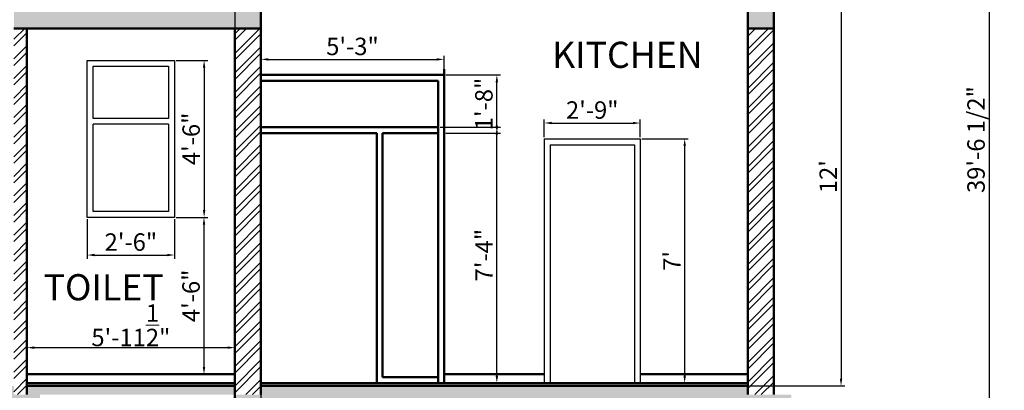
# Model space of a CAD drawing. Units: inches. Extents: x 1615 to 2231, y 1931 to 2519.
# Tile 5 of 6: x 1892 to 2231, y 2153 to 2281. Entities that reach past the tile are written whole.
import ezdxf

# ---------------------------------------------------------------- set-up
doc = ezdxf.new("R2010")
doc.units = ezdxf.units.IN
for name, color, linetype, lineweight in [('A-ANNO-DIMS', 2, 'Continuous', 18), ('A-AREA-IDEN', 7, 'Continuous', 25), ('A-DOOR', 3, 'Continuous', 25), ('A-GLAZ', 4, 'Continuous', 25), ('A-SECT', 7, 'Continuous', 50), ('A-WALL-PATT', 8, 'Continuous', 13)]:
    doc.layers.add(name, color=color, linetype=linetype, lineweight=lineweight)
doc.styles.get("Standard").update_dxf_attribs({"font": 'arial.ttf'})
doc.dimstyles.new('ISO-25', dxfattribs={"dimtxt": 6, "dimasz": 2.5, "dimexe": 1.25, "dimexo": 0.625, "dimtad": 1, "dimdec": 1, "dimlunit": 4, "dimtxsty": 'Standard', "dimcen": 2.5, "dimadec": 0, "dimazin": 0, "dimtfac": 1, "dimtdec": 1, "dimtmove": 0, "dimatfit": 3, "dimfxl": 1, "dimarcsym": 0})

# ---------------------------------------------------------------- blocks, each defined once
blk = doc.blocks.new('*D30')
at = {"layer": 'A-ANNO-DIMS', "color": 0, "lineweight": -2, "transparency": 16777216}
for p, q in [((1915.12, 2211.9), (1915.12, 2198.31)), ((1945.12, 2211.9), (1945.12, 2198.31)), ((1917.62, 2199.56), (1942.62, 2199.56))]:
    blk.add_line(p, q, dxfattribs=at)
at = {"layer": 'A-ANNO-DIMS', "color": 0, "lineweight": 100, "transparency": 16777216}
for points in [[(1917.62, 2199.98), (1917.62, 2199.14), (1915.12, 2199.56)], [(1942.62, 2199.98), (1942.62, 2199.14), (1945.12, 2199.56)]]:
    blk.add_solid(points, dxfattribs=at)
at = {"layer": 'Defpoints', "color": 0, "lineweight": 100, "transparency": 16777216}
for p in [(1915.12, 2212.53), (1945.12, 2212.53), (1945.12, 2199.56)]:
    blk.add_point(p, dxfattribs=at)
at = {"layer": 'A-ANNO-DIMS', "color": 0, "transparency": 16777216, "insert": (1930.12, 2203.25), "char_height": 6, "attachment_point": 5}
blk.add_mtext('2\'-6"', dxfattribs=at)
blk = doc.blocks.new('*D31')
at = {"layer": 'A-ANNO-DIMS', "color": 0, "lineweight": -2, "transparency": 16777216}
for p, q in [((1945.74, 2266.53), (1956.57, 2266.53)), ((1955.32, 2264.03), (1955.32, 2215.03)), ((1945.74, 2212.53), (1956.57, 2212.53))]:
    blk.add_line(p, q, dxfattribs=at)
at = {"layer": 'A-ANNO-DIMS', "color": 0, "lineweight": 100, "transparency": 16777216}
for points in [[(1954.91, 2264.03), (1955.74, 2264.03), (1955.32, 2266.53)], [(1954.91, 2215.03), (1955.74, 2215.03), (1955.32, 2212.53)]]:
    blk.add_solid(points, dxfattribs=at)
at = {"layer": 'Defpoints', "color": 0, "lineweight": 100, "transparency": 16777216}
for p in [(1945.12, 2266.53), (1945.12, 2212.53), (1955.32, 2212.53)]:
    blk.add_point(p, dxfattribs=at)
at = {"layer": 'A-ANNO-DIMS', "color": 0, "transparency": 16777216, "insert": (1951.63, 2239.53), "char_height": 6, "attachment_point": 5, "rotation": 90}
blk.add_mtext('4\'-6"', dxfattribs=at)
blk = doc.blocks.new('*D32')
at = {"layer": 'A-ANNO-DIMS', "color": 0, "lineweight": -2, "transparency": 16777216}
for p, q in [((1945.74, 2212.53), (1956.53, 2212.53)), ((1955.28, 2210.03), (1955.28, 2161.03)), ((1945.74, 2158.53), (1956.53, 2158.53))]:
    blk.add_line(p, q, dxfattribs=at)
at = {"layer": 'A-ANNO-DIMS', "color": 0, "lineweight": 100, "transparency": 16777216}
for points in [[(1954.87, 2210.03), (1955.7, 2210.03), (1955.28, 2212.53)], [(1954.87, 2161.03), (1955.7, 2161.03), (1955.28, 2158.53)]]:
    blk.add_solid(points, dxfattribs=at)
at = {"layer": 'Defpoints', "color": 0, "lineweight": 100, "transparency": 16777216}
for p in [(1945.12, 2212.53), (1945.12, 2158.53), (1955.28, 2158.53)]:
    blk.add_point(p, dxfattribs=at)
at = {"layer": 'A-ANNO-DIMS', "color": 0, "transparency": 16777216, "insert": (1951.6, 2185.53), "char_height": 6, "attachment_point": 5, "rotation": 90}
blk.add_mtext('4\'-6"', dxfattribs=at)
blk = doc.blocks.new('*D44')
at = {"layer": 'A-ANNO-DIMS', "color": 0, "lineweight": -2, "transparency": 16777216}
for p, q in [((2036.49, 2243.53), (2057.3, 2243.53)), ((2056.05, 2158.03), (2056.05, 2241.03)), ((2038.49, 2155.53), (2057.3, 2155.53))]:
    blk.add_line(p, q, dxfattribs=at)
at = {"layer": 'A-ANNO-DIMS', "color": 0, "lineweight": 100, "transparency": 16777216}
for points in [[(2055.63, 2241.03), (2056.47, 2241.03), (2056.05, 2243.53)], [(2055.63, 2158.03), (2056.47, 2158.03), (2056.05, 2155.53)]]:
    blk.add_solid(points, dxfattribs=at)
at = {"layer": 'Defpoints', "color": 0, "lineweight": 100, "transparency": 16777216}
for p in [(2035.87, 2243.53), (2056.05, 2243.53), (2037.87, 2155.53)]:
    blk.add_point(p, dxfattribs=at)
at = {"layer": 'A-ANNO-DIMS', "color": 0, "transparency": 16777216, "insert": (2052.43, 2199.53), "char_height": 6, "attachment_point": 5, "rotation": 90}
blk.add_mtext('7\'-4"', dxfattribs=at)
blk = doc.blocks.new('*D45')
at = {"layer": 'A-ANNO-DIMS', "color": 0, "lineweight": -2, "transparency": 16777216}
for p, q in [((1974.87, 2262.15), (1974.87, 2268.12)), ((1977.37, 2266.87), (2035.37, 2266.87)), ((2037.87, 2262.15), (2037.87, 2268.12))]:
    blk.add_line(p, q, dxfattribs=at)
at = {"layer": 'A-ANNO-DIMS', "color": 0, "lineweight": 100, "transparency": 16777216}
for points in [[(1977.37, 2267.29), (1977.37, 2266.46), (1974.87, 2266.87)], [(2035.37, 2267.29), (2035.37, 2266.46), (2037.87, 2266.87)]]:
    blk.add_solid(points, dxfattribs=at)
at = {"layer": 'Defpoints', "color": 0, "lineweight": 100, "transparency": 16777216}
for p in [(2037.87, 2266.87), (1974.87, 2261.53), (2037.87, 2261.53)]:
    blk.add_point(p, dxfattribs=at)
at = {"layer": 'A-ANNO-DIMS', "color": 0, "transparency": 16777216, "insert": (2006.37, 2270.56), "char_height": 6, "attachment_point": 5}
blk.add_mtext('5\'-3"', dxfattribs=at)
blk = doc.blocks.new('*D49')
at = {"layer": 'A-ANNO-DIMS', "color": 0, "lineweight": -2, "transparency": 16777216}
for p, q in [((2038.49, 2261.53), (2057.3, 2261.53)), ((2056.05, 2244.03), (2056.05, 2259.03)), ((2038.49, 2241.53), (2057.3, 2241.53))]:
    blk.add_line(p, q, dxfattribs=at)
at = {"layer": 'A-ANNO-DIMS', "color": 0, "lineweight": 100, "transparency": 16777216}
for points in [[(2055.63, 2259.03), (2056.47, 2259.03), (2056.05, 2261.53)], [(2055.63, 2244.03), (2056.47, 2244.03), (2056.05, 2241.53)]]:
    blk.add_solid(points, dxfattribs=at)
at = {"layer": 'Defpoints', "color": 0, "lineweight": 100, "transparency": 16777216}
for p in [(2037.87, 2261.53), (2056.05, 2261.53), (2037.87, 2241.53)]:
    blk.add_point(p, dxfattribs=at)
at = {"layer": 'A-ANNO-DIMS', "color": 0, "transparency": 16777216, "insert": (2052.36, 2251.53), "char_height": 6, "attachment_point": 5, "rotation": 90}
blk.add_mtext('1\'-8"', dxfattribs=at)
blk = doc.blocks.new('*D50')
at = {"layer": 'A-ANNO-DIMS', "color": 0, "lineweight": -2, "transparency": 16777216}
for p, q in [((1974.87, 2262.15), (1974.87, 2268.12)), ((1977.37, 2266.87), (2035.37, 2266.87)), ((2037.87, 2262.15), (2037.87, 2268.12))]:
    blk.add_line(p, q, dxfattribs=at)
at = {"layer": 'A-ANNO-DIMS', "color": 0, "lineweight": 100, "transparency": 16777216}
for points in [[(1977.37, 2267.29), (1977.37, 2266.46), (1974.87, 2266.87)], [(2035.37, 2267.29), (2035.37, 2266.46), (2037.87, 2266.87)]]:
    blk.add_solid(points, dxfattribs=at)
at = {"layer": 'Defpoints', "color": 0, "lineweight": 100, "transparency": 16777216}
for p in [(2037.87, 2266.87), (1974.87, 2261.53), (2037.87, 2261.53)]:
    blk.add_point(p, dxfattribs=at)
at = {"layer": 'A-ANNO-DIMS', "color": 0, "transparency": 16777216, "insert": (2006.37, 2270.56), "char_height": 6, "attachment_point": 5}
blk.add_mtext('5\'-3"', dxfattribs=at)
blk = doc.blocks.new('*D51')
at = {"layer": 'A-ANNO-DIMS', "color": 0, "lineweight": -2, "transparency": 16777216}
for p, q in [((2105.99, 2239.53), (2121.93, 2239.53)), ((2120.68, 2158.03), (2120.68, 2237.03)), ((2105.99, 2155.53), (2121.93, 2155.53))]:
    blk.add_line(p, q, dxfattribs=at)
at = {"layer": 'A-ANNO-DIMS', "color": 0, "lineweight": 100, "transparency": 16777216}
for points in [[(2120.27, 2237.03), (2121.1, 2237.03), (2120.68, 2239.53)], [(2120.27, 2158.03), (2121.1, 2158.03), (2120.68, 2155.53)]]:
    blk.add_solid(points, dxfattribs=at)
at = {"layer": 'Defpoints', "color": 0, "lineweight": 100, "transparency": 16777216}
for p in [(2105.37, 2239.53), (2120.68, 2239.53), (2105.37, 2155.53)]:
    blk.add_point(p, dxfattribs=at)
at = {"layer": 'A-ANNO-DIMS', "color": 0, "transparency": 16777216, "insert": (2117.06, 2197.53), "char_height": 6, "attachment_point": 5, "rotation": 90}
blk.add_mtext("7'", dxfattribs=at)
blk = doc.blocks.new('*D52')
at = {"layer": 'A-ANNO-DIMS', "color": 0, "lineweight": -2, "transparency": 16777216}
for p, q in [((2072.37, 2240.15), (2072.37, 2246.23)), ((2105.37, 2240.15), (2105.37, 2246.23)), ((2074.87, 2244.98), (2102.87, 2244.98))]:
    blk.add_line(p, q, dxfattribs=at)
at = {"layer": 'A-ANNO-DIMS', "color": 0, "lineweight": 100, "transparency": 16777216}
for points in [[(2074.87, 2245.4), (2074.87, 2244.57), (2072.37, 2244.98)], [(2102.87, 2245.4), (2102.87, 2244.57), (2105.37, 2244.98)]]:
    blk.add_solid(points, dxfattribs=at)
at = {"layer": 'Defpoints', "color": 0, "lineweight": 100, "transparency": 16777216}
for p in [(2105.37, 2244.98), (2072.37, 2239.53), (2105.37, 2239.53)]:
    blk.add_point(p, dxfattribs=at)
at = {"layer": 'A-ANNO-DIMS', "color": 0, "transparency": 16777216, "insert": (2088.87, 2248.67), "char_height": 6, "attachment_point": 5}
blk.add_mtext('2\'-9"', dxfattribs=at)
blk = doc.blocks.new('*D53')
at = {"layer": 'A-ANNO-DIMS', "color": 0, "lineweight": -2, "transparency": 16777216}
for p, q in [((2036.49, 2243.53), (2057.3, 2243.53)), ((2056.05, 2158.03), (2056.05, 2241.03)), ((2038.49, 2155.53), (2057.3, 2155.53))]:
    blk.add_line(p, q, dxfattribs=at)
at = {"layer": 'A-ANNO-DIMS', "color": 0, "lineweight": 100, "transparency": 16777216}
for points in [[(2055.63, 2241.03), (2056.47, 2241.03), (2056.05, 2243.53)], [(2055.63, 2158.03), (2056.47, 2158.03), (2056.05, 2155.53)]]:
    blk.add_solid(points, dxfattribs=at)
at = {"layer": 'Defpoints', "color": 0, "lineweight": 100, "transparency": 16777216}
for p in [(2035.87, 2243.53), (2056.05, 2243.53), (2037.87, 2155.53)]:
    blk.add_point(p, dxfattribs=at)
at = {"layer": 'A-ANNO-DIMS', "color": 0, "transparency": 16777216, "insert": (2052.43, 2199.53), "char_height": 6, "attachment_point": 5, "rotation": 90}
blk.add_mtext('7\'-4"', dxfattribs=at)
blk = doc.blocks.new('*D60')
at = {"layer": 'A-ANNO-DIMS', "color": 0, "lineweight": -2, "transparency": 16777216}
for p, q in [((1894.37, 2159.15), (1894.37, 2168.95)), ((1965.87, 2159.15), (1965.87, 2168.95)), ((1896.87, 2167.7), (1963.37, 2167.7))]:
    blk.add_line(p, q, dxfattribs=at)
at = {"layer": 'A-ANNO-DIMS', "color": 0, "lineweight": 100, "transparency": 16777216}
for points in [[(1896.87, 2168.12), (1896.87, 2167.28), (1894.37, 2167.7)], [(1963.37, 2168.12), (1963.37, 2167.28), (1965.87, 2167.7)]]:
    blk.add_solid(points, dxfattribs=at)
at = {"layer": 'Defpoints', "color": 0, "lineweight": 100, "transparency": 16777216}
for p in [(1965.87, 2167.7), (1894.37, 2158.53), (1965.87, 2158.53)]:
    blk.add_point(p, dxfattribs=at)
at = {"layer": 'A-ANNO-DIMS', "color": 0, "transparency": 16777216, "insert": (1930.12, 2175.4), "char_height": 6, "attachment_point": 5}
blk.add_mtext('5\'-11{\\H1x;\\S1/2;}"', dxfattribs=at)
blk = doc.blocks.new('*D63')
at = {"layer": 'A-ANNO-DIMS', "color": 0, "lineweight": -2, "transparency": 16777216}
for p, q in [((2142.99, 2298.53), (2175.73, 2298.53)), ((2174.48, 2296.03), (2174.48, 2157.03)), ((2142.99, 2154.53), (2175.73, 2154.53))]:
    blk.add_line(p, q, dxfattribs=at)
at = {"layer": 'A-ANNO-DIMS', "color": 0, "lineweight": 100, "transparency": 16777216}
for points in [[(2174.07, 2296.03), (2174.9, 2296.03), (2174.48, 2298.53)], [(2174.07, 2157.03), (2174.9, 2157.03), (2174.48, 2154.53)]]:
    blk.add_solid(points, dxfattribs=at)
at = {"layer": 'Defpoints', "color": 0, "lineweight": 100, "transparency": 16777216}
for p in [(2142.37, 2298.53), (2142.37, 2154.53), (2174.48, 2154.53)]:
    blk.add_point(p, dxfattribs=at)
at = {"layer": 'A-ANNO-DIMS', "color": 0, "transparency": 16777216, "insert": (2170.85, 2226.53), "char_height": 6, "attachment_point": 5, "rotation": 90}
blk.add_mtext("12'", dxfattribs=at)
blk = doc.blocks.new('WIN-TOILET')
for p, q in [((1915.12, 2410.53), (1945.12, 2410.53)), ((1915.12, 2356.53), (1915.12, 2410.53)), ((1945.12, 2410.53), (1945.12, 2390.53)), ((1917.12, 2408.53), (1943.12, 2408.53)), ((1917.12, 2390.53), (1917.12, 2408.53)), ((1943.12, 2408.53), (1943.12, 2390.53)), ((1943.12, 2390.53), (1917.12, 2390.53)), ((1943.12, 2388.53), (1917.12, 2388.53)), ((1917.12, 2358.53), (1917.12, 2388.53)), ((1943.12, 2388.53), (1943.12, 2358.53)), ((1945.12, 2390.53), (1945.12, 2356.53)), ((1943.12, 2358.53), (1917.12, 2358.53)), ((1945.12, 2356.53), (1915.12, 2356.53))]:
    blk.add_line(p, q)
blk = doc.blocks.new('DOOR-KITCHEN')
for p, q in [((2072.37, 2383.53), (2072.37, 2299.53)), ((2072.37, 2383.53), (2105.37, 2383.53)), ((2105.37, 2383.53), (2105.37, 2299.53)), ((2074.37, 2381.53), (2103.37, 2381.53)), ((2074.37, 2381.53), (2074.37, 2299.53)), ((2103.37, 2381.53), (2103.37, 2299.53))]:
    blk.add_line(p, q)
blk = doc.blocks.new('*D79')
at = {"layer": 'A-ANNO-DIMS', "color": 0, "lineweight": -2, "transparency": 16777216}
for p, q in [((2151.99, 2476.53), (2226.69, 2476.53)), ((2225.44, 2474.03), (2225.44, 2004.53)), ((2175.99, 2002.03), (2226.69, 2002.03))]:
    blk.add_line(p, q, dxfattribs=at)
at = {"layer": 'A-ANNO-DIMS', "color": 0, "lineweight": 100, "transparency": 16777216}
for points in [[(2225.02, 2474.03), (2225.86, 2474.03), (2225.44, 2476.53)], [(2225.02, 2004.53), (2225.86, 2004.53), (2225.44, 2002.03)]]:
    blk.add_solid(points, dxfattribs=at)
at = {"layer": 'Defpoints', "color": 0, "lineweight": 100, "transparency": 16777216}
for p in [(2151.37, 2476.53), (2175.37, 2002.03), (2225.44, 2002.03)]:
    blk.add_point(p, dxfattribs=at)
at = {"layer": 'A-ANNO-DIMS', "color": 0, "transparency": 16777216, "insert": (2221.71, 2239.28), "char_height": 6, "attachment_point": 5, "rotation": 90}
blk.add_mtext('39\'-6 1/2"', dxfattribs=at)
blk = doc.blocks.new('*D83')
at = {"layer": 'A-ANNO-DIMS', "color": 0, "lineweight": -2, "transparency": 16777216}
for p, q in [((1965.87, 2420.67), (1965.87, 1970.95)), ((1974.87, 2420.67), (1974.87, 1970.95)), ((1968.37, 1972.2), (1972.37, 1972.2)), ((1974.87, 1972.2), (1994.57, 1972.2))]:
    blk.add_line(p, q, dxfattribs=at)
at = {"layer": 'A-ANNO-DIMS', "color": 0, "lineweight": 100, "transparency": 16777216}
for points in [[(1968.37, 1972.62), (1968.37, 1971.78), (1965.87, 1972.2)], [(1972.37, 1972.62), (1972.37, 1971.78), (1974.87, 1972.2)]]:
    blk.add_solid(points, dxfattribs=at)
at = {"layer": 'Defpoints', "color": 0, "lineweight": 100, "transparency": 16777216}
for p in [(1965.87, 2421.29), (1974.87, 2421.29), (1974.87, 1972.2)]:
    blk.add_point(p, dxfattribs=at)
at = {"layer": 'A-ANNO-DIMS', "color": 0, "transparency": 16777216, "insert": (1985.97, 1975.89), "char_height": 6, "attachment_point": 5}
blk.add_mtext('0\'-9"', dxfattribs=at)

msp = doc.modelspace()

# ---------------------------------------------------------------- hatches: boundary and pattern name
at = {"layer": 'A-WALL-PATT'}
h = msp.add_hatch(dxfattribs=at)
h.set_pattern_fill('ANSI32', color=256, scale=0.5)
h.paths.add_polyline_path([(1676.87, 2421.53), (1667.87, 2421.53), (1667.87, 2295.53), (1676.87, 2295.53)])
h.paths.add_polyline_path([(1676.87, 2277.53), (1667.87, 2277.53), (1667.87, 2151.53), (1676.87, 2151.53)])
h.paths.add_polyline_path([(1676.87, 2476.53), (1667.87, 2476.53), (1667.87, 2439.53), (1676.87, 2439.53)])
h.paths.add_polyline_path([(1894.37, 2421.29), (1889.87, 2421.29), (1889.87, 2295.53), (1894.37, 2295.53)])
h.paths.add_polyline_path([(1974.87, 2421.29), (1965.87, 2421.29), (1965.87, 2295.53), (1974.87, 2295.53)])
h.paths.add_polyline_path([(2151.37, 2421.29), (2142.37, 2421.29), (2142.37, 2295.53), (2151.37, 2295.53)])
h.paths.add_polyline_path([(2151.37, 2476.53), (2142.37, 2476.53), (2142.37, 2442.53), (2151.37, 2442.53)])
h.paths.add_polyline_path([(1974.87, 2277.53), (1965.87, 2277.53), (1965.87, 2151.53), (1974.87, 2151.53)])
h.paths.add_polyline_path([(1974.87, 2133.53), (1965.87, 2133.53), (1965.87, 2060.03), (1974.87, 2060.03)])
h.paths.add_polyline_path([(2098.87, 2145.53), (2094.37, 2145.53), (2094.37, 2059.03), (2098.87, 2059.03)])
h = msp.add_hatch(dxfattribs=at)
h.set_pattern_fill('AR-CONC', color=256, scale=0.1)
h.paths.add_polyline_path([(1898.87, 2151.53), (1667.87, 2151.53), (1667.87, 2145.53), (1679.87, 2145.53), (1682.87, 2145.53), (1889.87, 2145.53), (1889.87, 2133.53), (1974.87, 2133.53), (1974.87, 2145.53), (2142.37, 2145.53), (2142.37, 2133.53), (2157.37, 2133.53), (2157.37, 2151.53), (2155.87, 2151.53), (2151.37, 2151.53), (1965.87, 2151.53), (1965.87, 2139.53), (1898.87, 2139.53)])
h.paths.add_polyline_path([(1898.87, 2295.53), (1667.87, 2295.53), (1667.87, 2277.53), (1676.87, 2277.53), (1676.87, 2289.53), (1889.87, 2289.53), (1889.87, 2277.53), (1974.87, 2277.53), (1974.87, 2289.53), (2142.37, 2289.53), (2142.37, 2277.53), (2151.37, 2277.53), (2151.37, 2295.53), (1965.87, 2295.53), (1965.87, 2283.53), (1898.87, 2283.53)])
h.paths.add_polyline_path([(2142.37, 2439.53), (1676.87, 2439.53), (1667.87, 2439.53), (1667.87, 2421.53), (1676.87, 2421.53), (1676.87, 2433.53), (1889.87, 2433.53), (1889.87, 2421.29), (1898.87, 2421.29), (1898.87, 2433.53), (1965.87, 2433.53), (1965.87, 2421.29), (1974.87, 2421.29), (1974.87, 2433.53), (2142.37, 2433.53)])
h = msp.add_hatch(dxfattribs=at)
h.set_pattern_fill('DOTS', color=256, scale=0.5)
h.paths.add_polyline_path([(2142.37, 2442.53), (1839.37, 2442.53), (1676.87, 2442.53), (1676.87, 2439.53), (2142.37, 2439.53)])
h.paths.add_polyline_path([(1889.87, 2298.53), (1676.87, 2298.53), (1676.87, 2295.53), (1889.87, 2295.53)])
h.paths.add_polyline_path([(2142.37, 2298.53), (1974.87, 2298.53), (1974.87, 2295.53), (2142.37, 2295.53)])
h.paths.add_polyline_path([(1889.87, 2154.53), (1676.87, 2154.53), (1676.87, 2151.53), (1889.87, 2151.53)])
h.paths.add_polyline_path([(1965.87, 2154.53), (1894.37, 2154.53), (1894.37, 2151.53), (1965.87, 2151.53)])
h.paths.add_polyline_path([(2142.37, 2154.53), (1974.87, 2154.53), (1974.87, 2151.53), (2142.37, 2151.53)])
h.paths.add_polyline_path([(2094.37, 2062.03), (1974.87, 2062.03), (1974.87, 2059.03), (2094.37, 2059.03)])
h.paths.add_polyline_path([(2142.37, 2062.03), (2098.87, 2062.03), (2098.87, 2059.03), (2142.37, 2059.03)])
h.paths.add_polyline_path([(1956.87, 2049.53), (1693.37, 2049.53), (1693.37, 2046.53), (1956.87, 2046.53)])
h = msp.add_hatch(dxfattribs=at)
h.set_pattern_fill('ANSI32', color=256, scale=0.5)
h.paths.add_polyline_path([(2151.37, 2277.53), (2142.37, 2277.53), (2142.37, 2151.53), (2151.37, 2151.53)])
h.paths.add_polyline_path([(1894.37, 2277.53), (1889.87, 2277.53), (1889.87, 2151.53), (1894.37, 2151.53)])

# ---------------------------------------------------------------- linework, layer by layer
at = {"layer": 'A-SECT'}
for p, q in [((2151.37, 2476.53), (2151.37, 2151.53)), ((1974.87, 2289.53), (1974.87, 2151.53)), ((2142.37, 2289.53), (2142.37, 2151.53)), ((1889.87, 2277.53), (1974.87, 2277.53)), ((1894.37, 2277.53), (1894.37, 2151.53)), ((1965.87, 2277.53), (1965.87, 2139.53)), ((2142.37, 2277.53), (2151.37, 2277.53)), ((2037.87, 2263.53), (2037.87, 2155.53)), ((1974.87, 2261.53), (2037.87, 2261.53)), ((1974.87, 2259.53), (2035.87, 2259.53)), ((2035.87, 2259.53), (2035.87, 2241.53)), ((1974.87, 2243.53), (2035.87, 2243.53)), ((1974.87, 2241.53), (2014.71, 2241.53)), ((2014.71, 2241.53), (2014.71, 2155.53)), ((2016.71, 2241.53), (2016.71, 2157.53)), ((2016.71, 2241.53), (2035.87, 2241.53)), ((2035.87, 2241.53), (2035.87, 2155.53)), ((1894.37, 2158.53), (1965.87, 2158.53)), ((2037.87, 2158.53), (2072.37, 2158.53)), ((2105.37, 2158.53), (2142.37, 2158.53)), ((1894.37, 2155.53), (1965.87, 2155.53)), ((1974.87, 2155.53), (2142.37, 2155.53)), ((2016.71, 2157.53), (2035.87, 2157.53)), ((1894.37, 2154.53), (1965.87, 2154.53)), ((1974.87, 2154.53), (2142.37, 2154.53))]:
    msp.add_line(p, q, dxfattribs=at)

# ---------------------------------------------------------------- block references
at = {"layer": 'A-DOOR'}
msp.add_blockref('DOOR-KITCHEN', (0, -144), dxfattribs=at)
at = {"layer": 'A-GLAZ'}
msp.add_blockref('WIN-TOILET', (0, -144), dxfattribs=at)

# ---------------------------------------------------------------- texts
at = {"layer": 'A-AREA-IDEN', "char_height": 9, "attachment_point": 1}
for s, width, insert in [('KITCHEN', 1.5481, (2075.08, 2272.94)), ('TOILET', 1.0394, (1900.1, 2192.98))]:
    msp.add_mtext_dynamic_manual_height_columns(s, width=width, gutter_width=12.5, heights=[0], dxfattribs=dict(at, insert=insert))

# ---------------------------------------------------------------- dimensions: what is measured, and where the dimension line sits
at = {"layer": 'A-ANNO-DIMS'}
for base, p1, p2, override, picture, middle in [((2225.44, 2002.03), (2151.37, 2476.53), (2175.37, 2002.03), {"dimdec": 1, "dimlfac": 1, "dimrnd": 0, "dimzin": 1, "dimdsep": 46, "dimlunit": 4, "dimfrac": 2}, '*D79', (2221.71, 2239.28)), ((2174.48, 2154.53), (2142.37, 2298.53), (2142.37, 2154.53), {"dimclrd": 0, "dimclre": 0, "dimclrt": 0}, '*D63', (2170.85, 2226.53)), ((1955.32, 2212.53), (1945.12, 2266.53), (1945.12, 2212.53), {"dimclrd": 0, "dimclre": 0, "dimclrt": 0}, '*D31', (1951.63, 2239.53)), ((2056.05, 2261.53), (2037.87, 2241.53), (2037.87, 2261.53), {"dimclrd": 0, "dimclre": 0, "dimclrt": 0}, '*D49', (2052.36, 2251.53)), ((2056.05, 2243.53), (2037.87, 2155.53), (2035.87, 2243.53), {"dimclrd": 0, "dimclre": 0, "dimclrt": 0}, '*D44', (2052.43, 2199.53)), ((2056.05, 2243.53), (2037.87, 2155.53), (2035.87, 2243.53), {"dimclrd": 0, "dimclre": 0, "dimclrt": 0}, '*D53', (2052.43, 2199.53)), ((2120.68, 2239.53), (2105.37, 2155.53), (2105.37, 2239.53), {"dimclrd": 0, "dimclre": 0, "dimclrt": 0}, '*D51', (2117.06, 2197.53)), ((1955.28, 2158.53), (1945.12, 2212.53), (1945.12, 2158.53), {"dimclrd": 0, "dimclre": 0, "dimclrt": 0}, '*D32', (1951.6, 2185.53))]:
    dim = msp.add_linear_dim(base=base, p1=p1, p2=p2, angle=90, dimstyle='ISO-25', override=override, dxfattribs=at)
    dim.commit()
    dim.dimension.update_dxf_attribs({"geometry": picture, "text_midpoint": middle})
for base, p1, p2, override, picture, middle in [((1974.87, 1972.2), (1965.87, 2421.29), (1974.87, 2421.29), {"dimdec": 1, "dimlfac": 1, "dimrnd": 0, "dimzin": 1, "dimdsep": 46, "dimlunit": 4, "dimfrac": 2}, '*D83', (1985.97, 1975.89)), ((2037.87, 2266.87), (1974.87, 2261.53), (2037.87, 2261.53), {"dimclrd": 0, "dimclre": 0, "dimclrt": 0}, '*D45', (2006.37, 2270.56)), ((2037.87, 2266.87), (1974.87, 2261.53), (2037.87, 2261.53), {"dimclrd": 0, "dimclre": 0, "dimclrt": 0}, '*D50', (2006.37, 2270.56)), ((2105.37, 2244.98), (2072.37, 2239.53), (2105.37, 2239.53), {"dimclrd": 0, "dimclre": 0, "dimclrt": 0}, '*D52', (2088.87, 2248.67)), ((1945.12, 2199.56), (1915.12, 2212.53), (1945.12, 2212.53), {"dimclrd": 0, "dimclre": 0, "dimclrt": 0}, '*D30', (1930.12, 2203.25)), ((1965.87, 2167.7), (1894.37, 2158.53), (1965.87, 2158.53), {"dimclrd": 0, "dimclre": 0, "dimclrt": 0}, '*D60', (1930.12, 2175.4))]:
    dim = msp.add_linear_dim(base=base, p1=p1, p2=p2, dimstyle='ISO-25', override=override, dxfattribs=at)
    dim.commit()
    dim.dimension.update_dxf_attribs({"geometry": picture, "text_midpoint": middle})

doc.saveas('drawing.dxf')
